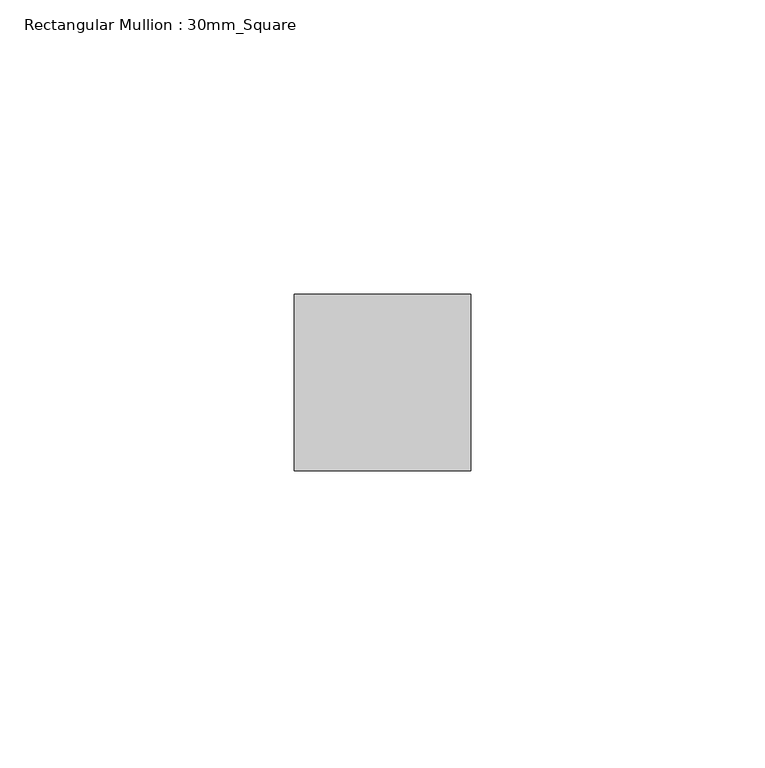
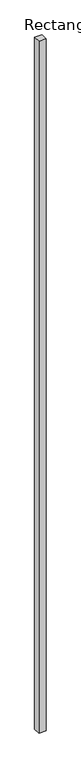
"""IFC4 building model written with IfcOpenShell, lengths in millimetres: member geometry, Rectangular Mullion : 30mm_Square."""

from ifc_helpers import new_model, si_unit, frame, origin, place, context, project, spatial, polyline, outline, extrude, source, transform, mapped, element, save


def rectangular_mullion_30mm_square_4b8855c0(model_context):
    return source(origin(), model_context, "Body", "SweptSolid", [
        extrude(outline(polyline([(0.0, 15.0), (0.0, -15.0), (-30.0, -15.0), (-30.0, 15.0), (0.0, 15.0)])), frame((0.0, 0.0, -3086.4985113), z_axis=(0.0, 0.0, 1.0), x_axis=(1.0, 0.0, 0.0)), (0.0, 0.0, 1.0), 3086.4985113),
    ])


if __name__ == "__main__":
    model = new_model("IFC4")
    model_context = context("Model", 3, world=origin())
    ifc_project = project(units=[si_unit("LENGTHUNIT", "METRE", prefix="MILLI")], contexts=[model_context])
    site = spatial("IfcSite", under=ifc_project)
    building = spatial("IfcBuilding", under=site)
    placement = place(None, origin())
    rectangular_mullion_30mm_square_shape = rectangular_mullion_30mm_square_4b8855c0(model_context)
    element("IfcMember", 1, ObjectType="Rectangular Mullion : 30mm_Square", at=placement, inside=building, context=model_context, shape_type="MappedRepresentation", body=[
        mapped(rectangular_mullion_30mm_square_shape, transform((0.0, 0.0, 0.0), x_axis=(1.0, 0.0, 0.0), y_axis=(0.0, 1.0, 0.0), z_axis=(0.0, 0.0, 1.0))),
    ])
    save(model, "model.ifc")

# Revit data of these elements
# Type "Rectangular Mullion : 30mm_Square"
#   Keynote = "H11"
#   built-in parameter 1007304 = 0.0984252 (stored number, unit not read)
#   built-in parameter 1007301 = 0.0492126 (stored number, unit not read)
#   built-in parameter 1007300 = 0.0492126 (stored number, unit not read)
# Element 1 (IfcMember, "Rectangular Mullion : 30mm_Square")
#   Materials on its faces: "Aluminium"
# Materials
#   "Aluminium": class "Metal", colour RGB 247 247 247, transparency 0, Description = "Aluminium 6061", Cost = 0
